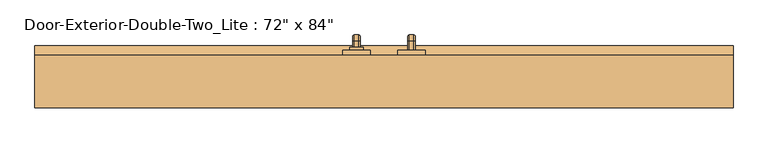
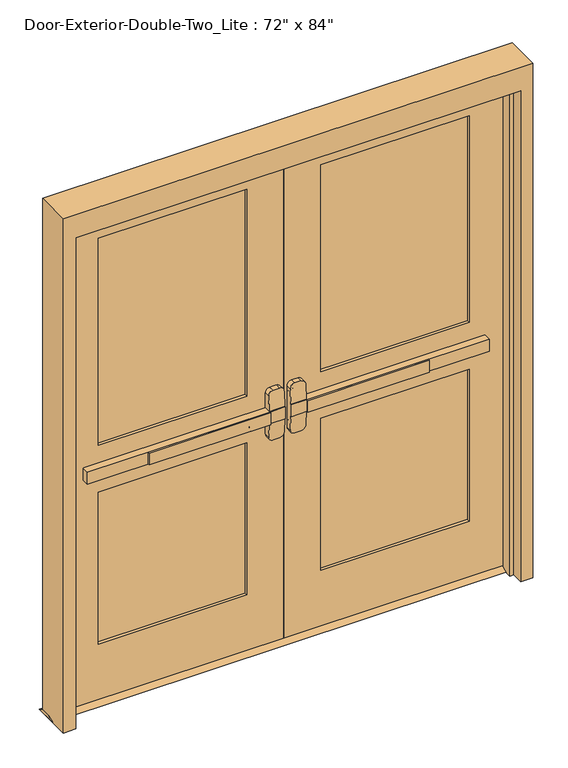
"""IFC4 building model written with IfcOpenShell, lengths in millimetres: door geometry."""

from ifc_helpers import new_model, si_unit, point, frame, frame_2d, origin, place, context, project, spatial, polyline, circle_curve, ellipse_curve, trimmed, segment, composite_curve, outline, extrude, faceted_brep, source, transform, mapped, element, save
from ifc_brep_helpers import plane_surface, cylinder_surface, revolved_surface, advanced_brep


def door_6260e01d(model_context):
    return source(origin(), model_context, "Body", "SolidModel", [
        extrude(outline(polyline([(-575.7333333, 0.0), (-575.7333333, 6.35), (-76.2, 6.35), (-76.2, 0.0), (-575.7333333, 0.0)])), frame((0.0, 0.0, 990.6), z_axis=(0.0, 0.0, 1.0), x_axis=(1.0, 0.0, 0.0)), (0.0, 0.0, 1.0), 50.8),
        advanced_brep(
        [(-12.7, 6.35, 1041.4), (-76.2, 6.35, 1041.4), (-825.5, 6.35, 1041.4), (-825.5, 6.35, 990.6), (-76.2, 6.35, 990.6), (-12.7, 6.35, 990.6), (-825.5, 38.1, 1041.4), (-76.2, 38.1, 1041.4), (-76.2, 38.1, 1104.9), (-57.15, 38.1, 1123.95), (-31.75, 38.1, 1123.95), (-12.7, 38.1, 1104.9), (-12.7, 38.1, 927.1), (-31.75, 38.1, 908.05), (-57.15, 38.1, 908.05), (-76.2, 38.1, 927.1), (-76.2, 38.1, 990.6), (-825.5, 38.1, 990.6), (-12.7, 9.5252467, 1041.4), (-76.2, 9.5252467, 1041.4), (-12.7, 9.5252467, 990.6), (-12.7, 14.5354269, 927.1), (-12.7, 14.5354269, 1104.9), (-76.2, 9.5252467, 990.6), (-76.2, 14.5354269, 1104.9), (-76.2, 14.5354269, 927.1), (-57.15, 16.038481, 1123.95), (-31.75, 16.038481, 1123.95), (-31.75, 16.038481, 908.05), (-57.15, 16.038481, 908.05)],
        [
            (0, 1),
            (1, 2),
            (2, 3),
            (3, 4),
            (4, 5),
            (5, 0),
            (6, 7),
            (7, 8),
            (8, 9, circle_curve(frame((-57.15, 38.1, 1104.9), z_axis=(0.0, 1.0, 0.0), x_axis=(-1.0, 0.0, 0.0)), 19.05)),
            (9, 10),
            (10, 11, circle_curve(frame((-31.75, 38.1, 1104.9), z_axis=(0.0, 1.0, 0.0), x_axis=(-1.0, 0.0, 0.0)), 19.05)),
            (11, 12),
            (12, 13, circle_curve(frame((-31.75, 38.1, 927.1), z_axis=(0.0, 1.0, 0.0), x_axis=(-1.0, 0.0, 0.0)), 19.05)),
            (13, 14),
            (14, 15, circle_curve(frame((-57.15, 38.1, 927.1), z_axis=(0.0, 1.0, 0.0), x_axis=(-1.0, 0.0, 0.0)), 19.05)),
            (15, 16),
            (16, 17),
            (17, 6),
            (0, 18),
            (18, 19),
            (19, 7),
            (6, 2),
            (5, 20),
            (20, 21),
            (21, 12),
            (11, 22),
            (22, 18),
            (16, 23),
            (23, 20),
            (3, 17),
            (19, 24),
            (24, 8),
            (15, 25),
            (25, 23),
            (9, 26),
            (26, 27),
            (27, 10),
            (13, 28),
            (28, 29),
            (29, 14),
            (29, 25, ellipse_curve(frame((-57.15, 14.5354269, 927.1), z_axis=(0.0, 0.9969018152893365, 0.07865602756830282), x_axis=(0.0, -0.07865602756830208, 0.9969018152893365)), 19.1092038, 19.05)),
            (24, 26, ellipse_curve(frame((-57.15, 14.5354269, 1104.9), z_axis=(0.0, 0.9969018152893376, -0.07865602756828934), x_axis=(0.0, -0.078656027568288, -0.9969018152893377)), 19.1092038, 19.05)),
            (27, 22, ellipse_curve(frame((-31.75, 14.5354269, 1104.9), z_axis=(0.0, 0.9969018152893376, -0.07865602756828934), x_axis=(0.0, -0.078656027568288, -0.9969018152893377)), 19.1092038, 19.05)),
            (21, 28, ellipse_curve(frame((-31.75, 14.5354269, 927.1), z_axis=(0.0, 0.9969018152893365, 0.07865602756830282), x_axis=(0.0, -0.07865602756830208, 0.9969018152893365)), 19.1092038, 19.05)),
        ],
        [
            plane_surface(frame((-12.7, 6.35, 1041.4), z_axis=(0.0, -1.0, 0.0), x_axis=(1.0, 0.0, 0.0))),
            plane_surface(frame((-12.7, 38.1, 1041.4), z_axis=(0.0, 1.0, 0.0), x_axis=(-1.0, 0.0, 0.0))),
            plane_surface(frame((-825.5, 6.35, 1041.4), z_axis=(0.0, 0.0, 1.0), x_axis=(0.0, 1.0, 0.0))),
            plane_surface(frame((-12.7, 6.35, 1041.4), z_axis=(1.0, 0.0, 0.0), x_axis=(0.0, 1.0, 0.0))),
            plane_surface(frame((-12.7, 6.35, 990.6), z_axis=(0.0, 0.0, -1.0), x_axis=(0.0, 1.0, 0.0))),
            plane_surface(frame((-825.5, 6.35, 990.6), z_axis=(-1.0, 0.0, 0.0), x_axis=(0.0, 1.0, 0.0))),
            plane_surface(frame((-76.2, 9.5252467, 927.1), z_axis=(-1.0, 0.0, 0.0), x_axis=(0.0, 1.0, 0.0))),
            plane_surface(frame((-57.15, 9.5252467, 1123.95), z_axis=(0.0, 0.0, 1.0), x_axis=(0.0, 1.0, 0.0))),
            plane_surface(frame((-31.75, 9.5252467, 908.05), z_axis=(0.0, 0.0, -1.0), x_axis=(0.0, 1.0, 0.0))),
            cylinder_surface(frame((-57.15, 38.1, 927.1), z_axis=(0.0, -1.0, 0.0), x_axis=(-1.0, 0.0, 0.0)), 19.05),
            cylinder_surface(frame((-57.15, 38.1, 1104.9), z_axis=(0.0, -1.0, 0.0), x_axis=(-1.0, 0.0, 0.0)), 19.05),
            cylinder_surface(frame((-31.75, 38.1, 1104.9), z_axis=(0.0, -1.0, 0.0), x_axis=(-1.0, 0.0, 0.0)), 19.05),
            cylinder_surface(frame((-31.75, 38.1, 927.1), z_axis=(0.0, -1.0, 0.0), x_axis=(-1.0, 0.0, 0.0)), 19.05),
            plane_surface(frame((-76.2, 9.5252467, 1041.4), z_axis=(0.0, -0.9969018152893376, 0.07865602756828934), x_axis=(1.0, 0.0, 0.0))),
            plane_surface(frame((-76.2, 16.038481, 908.05), z_axis=(0.0, -0.9969018152893365, -0.07865602756830282), x_axis=(1.0, 0.0, 0.0))),
        ],
        [
            (0, [[1, 2, 3, 4, 5, 6]]),
            (1, [[7, 8, 9, 10, 11, 12, 13, 14, 15, 16, 17, 18]]),
            (2, [[-2, -1, 19, 20, 21, -7, 22]]),
            (3, [[23, 24, 25, -12, 26, 27, -19, -6]]),
            (4, [[-17, 28, 29, -23, -5, -4, 30]]),
            (5, [[-22, -18, -30, -3]]),
            (6, [[-21, 31, 32, -8]]),
            (6, [[33, 34, -28, -16]]),
            (7, [[35, 36, 37, -10]]),
            (8, [[38, 39, 40, -14]]),
            (9, [[-40, 41, -33, -15]]),
            (10, [[-32, 42, -35, -9]]),
            (11, [[-37, 43, -26, -11]]),
            (12, [[-25, 44, -38, -13]]),
            (13, [[-27, -43, -36, -42, -31, -20]]),
            (14, [[-29, -34, -41, -39, -44, -24]]),
        ],
    ),
        extrude(outline(polyline([(82.55, 12.7), (107.95, 0.0), (12.7, 0.0), (38.1, 12.7), (82.55, 12.7)])), frame((-965.2, 0.0, 0.0), z_axis=(1.0, 0.0, 0.0), x_axis=(0.0, 1.0, 0.0)), (0.0, 0.0, 1.0), 1930.4),
        extrude(outline(polyline([(575.7333333, 0.0), (76.2, 0.0), (76.2, 6.35), (575.7333333, 6.35), (575.7333333, 0.0)])), frame((0.0, 0.0, 990.6), z_axis=(0.0, 0.0, 1.0), x_axis=(1.0, 0.0, 0.0)), (0.0, 0.0, 1.0), 50.8),
        advanced_brep(
        [(12.7, 6.35, 1041.4), (12.7, 6.35, 990.6), (76.2, 6.35, 990.6), (825.5, 6.35, 990.6), (825.5, 6.35, 1041.4), (76.2, 6.35, 1041.4), (825.5, 38.1, 1041.4), (825.5, 38.1, 990.6), (76.2, 38.1, 990.6), (76.2, 38.1, 927.1), (57.15, 38.1, 908.05), (31.75, 38.1, 908.05), (12.7, 38.1, 927.1), (12.7, 38.1, 1104.9), (31.75, 38.1, 1123.95), (57.15, 38.1, 1123.95), (76.2, 38.1, 1104.9), (76.2, 38.1, 1041.4), (76.2, 9.5252467, 1041.4), (12.7, 9.5252467, 1041.4), (12.7, 14.5354269, 1104.9), (12.7, 14.5354269, 927.1), (12.7, 9.5252467, 990.6), (76.2, 9.5252467, 990.6), (76.2, 14.5354269, 927.1), (76.2, 14.5354269, 1104.9), (31.75, 16.038481, 1123.95), (57.15, 16.038481, 1123.95), (57.15, 16.038481, 908.05), (31.75, 16.038481, 908.05)],
        [
            (0, 1),
            (1, 2),
            (2, 3),
            (3, 4),
            (4, 5),
            (5, 0),
            (6, 7),
            (7, 8),
            (8, 9),
            (9, 10, circle_curve(frame((57.15, 38.1, 927.1), z_axis=(0.0, 1.0, 0.0), x_axis=(1.0, 0.0, 0.0)), 19.05)),
            (10, 11),
            (11, 12, circle_curve(frame((31.75, 38.1, 927.1), z_axis=(0.0, 1.0, 0.0), x_axis=(1.0, 0.0, 0.0)), 19.05)),
            (12, 13),
            (13, 14, circle_curve(frame((31.75, 38.1, 1104.9), z_axis=(0.0, 1.0, 0.0), x_axis=(1.0, 0.0, 0.0)), 19.05)),
            (14, 15),
            (15, 16, circle_curve(frame((57.15, 38.1, 1104.9), z_axis=(0.0, 1.0, 0.0), x_axis=(1.0, 0.0, 0.0)), 19.05)),
            (16, 17),
            (17, 6),
            (4, 6),
            (17, 18),
            (18, 19),
            (19, 0),
            (19, 20),
            (20, 13),
            (12, 21),
            (21, 22),
            (22, 1),
            (7, 3),
            (22, 23),
            (23, 8),
            (23, 24),
            (24, 9),
            (16, 25),
            (25, 18),
            (14, 26),
            (26, 27),
            (27, 15),
            (10, 28),
            (28, 29),
            (29, 11),
            (24, 28, ellipse_curve(frame((57.15, 14.5354269, 927.1), z_axis=(0.0, 0.9969018152893365, 0.07865602756830282), x_axis=(0.0, -0.07865602756830208, 0.9969018152893365)), 19.1092038, 19.05)),
            (27, 25, ellipse_curve(frame((57.15, 14.5354269, 1104.9), z_axis=(0.0, 0.9969018152893376, -0.07865602756828934), x_axis=(0.0, -0.078656027568288, -0.9969018152893377)), 19.1092038, 19.05)),
            (20, 26, ellipse_curve(frame((31.75, 14.5354269, 1104.9), z_axis=(0.0, 0.9969018152893376, -0.07865602756828934), x_axis=(0.0, -0.078656027568288, -0.9969018152893377)), 19.1092038, 19.05)),
            (29, 21, ellipse_curve(frame((31.75, 14.5354269, 927.1), z_axis=(0.0, 0.9969018152893365, 0.07865602756830282), x_axis=(0.0, -0.07865602756830208, 0.9969018152893365)), 19.1092038, 19.05)),
        ],
        [
            plane_surface(frame((12.7, 6.35, 1041.4), z_axis=(0.0, -1.0, 0.0), x_axis=(-1.0, 0.0, 0.0))),
            plane_surface(frame((12.7, 38.1, 1041.4), z_axis=(0.0, 1.0, 0.0), x_axis=(1.0, 0.0, 0.0))),
            plane_surface(frame((825.5, 6.35, 1041.4), z_axis=(0.0, 0.0, 1.0), x_axis=(0.0, 1.0, 0.0))),
            plane_surface(frame((12.7, 6.35, 1041.4), z_axis=(-1.0, 0.0, 0.0), x_axis=(0.0, 1.0, 0.0))),
            plane_surface(frame((12.7, 6.35, 990.6), z_axis=(0.0, 0.0, -1.0), x_axis=(0.0, 1.0, 0.0))),
            plane_surface(frame((825.5, 6.35, 990.6), z_axis=(1.0, 0.0, 0.0), x_axis=(0.0, 1.0, 0.0))),
            plane_surface(frame((76.2, 9.5252467, 927.1), z_axis=(1.0, 0.0, 0.0), x_axis=(0.0, 1.0, 0.0))),
            plane_surface(frame((57.15, 9.5252467, 1123.95), z_axis=(0.0, 0.0, 1.0), x_axis=(0.0, 1.0, 0.0))),
            plane_surface(frame((31.75, 9.5252467, 908.05), z_axis=(0.0, 0.0, -1.0), x_axis=(0.0, 1.0, 0.0))),
            cylinder_surface(frame((57.15, 38.1, 927.1), z_axis=(0.0, -1.0, 0.0), x_axis=(1.0, 0.0, 0.0)), 19.05),
            cylinder_surface(frame((57.15, 38.1, 1104.9), z_axis=(0.0, -1.0, 0.0), x_axis=(1.0, 0.0, 0.0)), 19.05),
            cylinder_surface(frame((31.75, 38.1, 1104.9), z_axis=(0.0, -1.0, 0.0), x_axis=(1.0, 0.0, 0.0)), 19.05),
            cylinder_surface(frame((31.75, 38.1, 927.1), z_axis=(0.0, -1.0, 0.0), x_axis=(1.0, 0.0, 0.0)), 19.05),
            plane_surface(frame((76.2, 9.5252467, 1041.4), z_axis=(0.0, -0.9969018152893376, 0.07865602756828934), x_axis=(-1.0, 0.0, 0.0))),
            plane_surface(frame((76.2, 16.038481, 908.05), z_axis=(0.0, -0.9969018152893365, -0.07865602756830282), x_axis=(-1.0, 0.0, 0.0))),
        ],
        [
            (0, [[1, 2, 3, 4, 5, 6]]),
            (1, [[7, 8, 9, 10, 11, 12, 13, 14, 15, 16, 17, 18]]),
            (2, [[19, -18, 20, 21, 22, -6, -5]]),
            (3, [[-1, -22, 23, 24, -13, 25, 26, 27]]),
            (4, [[28, -3, -2, -27, 29, 30, -8]]),
            (5, [[-4, -28, -7, -19]]),
            (6, [[-9, -30, 31, 32]]),
            (6, [[-17, 33, 34, -20]]),
            (7, [[-15, 35, 36, 37]]),
            (8, [[-11, 38, 39, 40]]),
            (9, [[-10, -32, 41, -38]]),
            (10, [[-16, -37, 42, -33]]),
            (11, [[-14, -24, 43, -35]]),
            (12, [[-12, -40, 44, -25]]),
            (13, [[-21, -34, -42, -36, -43, -23]]),
            (14, [[-26, -44, -39, -41, -31, -29]]),
        ],
    ),
        advanced_brep(
        [(66.2, 95.25, 1017.190625), (66.2, 95.25, 1014.809375), (69.771875, 95.25, 1011.2375), (82.6284594, 95.25, 1011.2375), (86.2, 95.25, 1014.8090406), (86.2, 95.25, 1017.190625), (82.628125, 95.25, 1020.7625), (69.771875, 95.25, 1020.7625), (66.2, 95.25, 887.809375), (69.771875, 95.25, 884.2375), (82.628125, 95.25, 884.2375), (86.2, 95.25, 887.809375), (86.2, 95.25, 890.1909594), (82.6284594, 95.25, 893.7625), (69.771875, 95.25, 893.7625), (66.2, 95.25, 890.190625), (66.2, 120.65, 1017.190625), (66.2, 134.540625, 1003.3), (66.2, 134.540625, 901.7), (66.2, 120.65, 887.809375), (66.2, 120.65, 890.190625), (66.2, 132.159375, 901.7), (66.2, 132.159375, 1003.3), (66.2, 120.65, 1014.809375), (69.771875, 120.65, 1011.2375), (82.6284594, 120.65, 1011.2375), (86.2, 120.65, 1014.8090406), (86.2, 132.1590406, 1003.3), (86.2, 132.1590406, 901.7), (86.2, 120.65, 890.1909594), (86.2, 120.65, 887.809375), (86.2, 134.540625, 901.7), (86.2, 134.540625, 1003.3), (86.2, 120.65, 1017.190625), (82.628125, 120.65, 1020.7625), (69.771875, 120.65, 1020.7625), (69.771875, 128.5875, 1003.3), (82.6284594, 128.5875, 1003.3), (82.628125, 138.1125, 1003.3), (69.771875, 138.1125, 1003.3), (69.771875, 128.5875, 901.7), (82.6284594, 128.5875, 901.7), (82.628125, 138.1125, 901.7), (69.771875, 138.1125, 901.7), (69.771875, 120.65, 893.7625), (82.6284594, 120.65, 893.7625), (82.628125, 120.65, 884.2375), (69.771875, 120.65, 884.2375)],
        [
            (0, 1),
            (1, 2, circle_curve(frame((69.771875, 95.25, 1014.809375), z_axis=(0.0, -1.0, 0.0), x_axis=(0.0, 0.0, 1.0)), 3.571875)),
            (2, 3),
            (3, 4, circle_curve(frame((82.6284594, 95.25, 1014.8090406), z_axis=(0.0, -1.0, 0.0), x_axis=(0.0, 0.0, 1.0)), 3.5715406)),
            (4, 5),
            (5, 6, circle_curve(frame((82.628125, 95.25, 1017.190625), z_axis=(0.0, -1.0, 0.0), x_axis=(0.0, 0.0, 1.0)), 3.571875)),
            (6, 7),
            (7, 0, circle_curve(frame((69.771875, 95.25, 1017.190625), z_axis=(0.0, -1.0, 0.0), x_axis=(0.0, 0.0, 1.0)), 3.571875)),
            (8, 9, circle_curve(frame((69.771875, 95.25, 887.809375), z_axis=(0.0, -1.0, 0.0), x_axis=(0.0, 0.0, -1.0)), 3.571875)),
            (9, 10),
            (10, 11, circle_curve(frame((82.628125, 95.25, 887.809375), z_axis=(0.0, -1.0, 0.0), x_axis=(0.0, 0.0, -1.0)), 3.571875)),
            (11, 12),
            (12, 13, circle_curve(frame((82.6284594, 95.25, 890.1909594), z_axis=(0.0, -1.0, 0.0), x_axis=(0.0, 0.0, -1.0)), 3.5715406)),
            (13, 14),
            (14, 15, circle_curve(frame((69.771875, 95.25, 890.190625), z_axis=(0.0, -1.0, 0.0), x_axis=(0.0, 0.0, -1.0)), 3.571875)),
            (15, 8),
            (0, 16),
            (16, 17, circle_curve(frame((66.2, 120.65, 1003.3), z_axis=(-1.0, 0.0, 0.0), x_axis=(0.0, 0.0, 1.0)), 13.890625)),
            (17, 18),
            (18, 19, circle_curve(frame((66.2, 120.65, 901.7), z_axis=(-1.0, 0.0, 0.0), x_axis=(0.0, 1.0, 0.0)), 13.890625)),
            (19, 8),
            (15, 20),
            (20, 21, circle_curve(frame((66.2, 120.65, 901.7), z_axis=(1.0, 0.0, 0.0), x_axis=(0.0, 1.0, 0.0)), 11.509375)),
            (21, 22),
            (22, 23, circle_curve(frame((66.2, 120.65, 1003.3), z_axis=(1.0, 0.0, 0.0), x_axis=(0.0, 0.0, 1.0)), 11.509375)),
            (23, 1),
            (23, 24, circle_curve(frame((69.771875, 120.65, 1014.809375), z_axis=(0.0, -1.0, 0.0), x_axis=(0.0, 0.0, 1.0)), 3.571875)),
            (24, 2),
            (24, 25),
            (25, 3),
            (25, 26, circle_curve(frame((82.6284594, 120.65, 1014.8090406), z_axis=(0.0, -1.0, 0.0), x_axis=(0.0, 0.0, 1.0)), 3.5715406)),
            (26, 4),
            (26, 27, circle_curve(frame((86.2, 120.65, 1003.3), z_axis=(-1.0, 0.0, 0.0), x_axis=(0.0, 0.0, 1.0)), 11.5090406)),
            (27, 28),
            (28, 29, circle_curve(frame((86.2, 120.65, 901.7), z_axis=(-1.0, 0.0, 0.0), x_axis=(0.0, 1.0, 0.0)), 11.5090406)),
            (29, 12),
            (11, 30),
            (30, 31, circle_curve(frame((86.2, 120.65, 901.7), z_axis=(1.0, 0.0, 0.0), x_axis=(0.0, 1.0, 0.0)), 13.890625)),
            (31, 32),
            (32, 33, circle_curve(frame((86.2, 120.65, 1003.3), z_axis=(1.0, 0.0, 0.0), x_axis=(0.0, 0.0, 1.0)), 13.890625)),
            (33, 5),
            (33, 34, circle_curve(frame((82.628125, 120.65, 1017.190625), z_axis=(0.0, -1.0, 0.0), x_axis=(0.0, 0.0, 1.0)), 3.571875)),
            (34, 6),
            (34, 35),
            (35, 7),
            (35, 16, circle_curve(frame((69.771875, 120.65, 1017.190625), z_axis=(0.0, -1.0, 0.0), x_axis=(0.0, 0.0, 1.0)), 3.571875)),
            (36, 24, circle_curve(frame((69.771875, 120.65, 1003.3), z_axis=(1.0, 0.0, 0.0), x_axis=(0.0, 0.0, 1.0)), 7.9375)),
            (22, 36, circle_curve(frame((69.771875, 132.159375, 1003.3), z_axis=(0.0, 0.0, 1.0), x_axis=(0.0, 1.0, 0.0)), 3.571875)),
            (37, 25, circle_curve(frame((82.6284594, 120.65, 1003.3), z_axis=(1.0, 0.0, 0.0), x_axis=(0.0, 0.0, 1.0)), 7.9375)),
            (36, 37),
            (37, 27, circle_curve(frame((82.6284594, 132.1590406, 1003.3), z_axis=(0.0, 0.0, 1.0), x_axis=(0.0, 1.0, 0.0)), 3.5715406)),
            (38, 34, circle_curve(frame((82.628125, 120.65, 1003.3), z_axis=(1.0, 0.0, 0.0), x_axis=(0.0, 0.0, 1.0)), 17.4625)),
            (32, 38, circle_curve(frame((82.628125, 134.540625, 1003.3), z_axis=(0.0, 0.0, 1.0), x_axis=(0.0, 1.0, 0.0)), 3.571875)),
            (39, 35, circle_curve(frame((69.771875, 120.65, 1003.3), z_axis=(1.0, 0.0, 0.0), x_axis=(0.0, 0.0, 1.0)), 17.4625)),
            (38, 39),
            (39, 17, circle_curve(frame((69.771875, 134.540625, 1003.3), z_axis=(0.0, 0.0, 1.0), x_axis=(0.0, 1.0, 0.0)), 3.571875)),
            (21, 40, circle_curve(frame((69.771875, 132.159375, 901.7), z_axis=(0.0, 0.0, 1.0), x_axis=(0.0, 1.0, 0.0)), 3.571875)),
            (40, 36),
            (40, 41),
            (41, 37),
            (41, 28, circle_curve(frame((82.6284594, 132.1590406, 901.7), z_axis=(0.0, 0.0, 1.0), x_axis=(0.0, 1.0, 0.0)), 3.5715406)),
            (31, 42, circle_curve(frame((82.628125, 134.540625, 901.7), z_axis=(0.0, 0.0, 1.0), x_axis=(0.0, 1.0, 0.0)), 3.571875)),
            (42, 38),
            (42, 43),
            (43, 39),
            (43, 18, circle_curve(frame((69.771875, 134.540625, 901.7), z_axis=(0.0, 0.0, 1.0), x_axis=(0.0, 1.0, 0.0)), 3.571875)),
            (44, 40, circle_curve(frame((69.771875, 120.65, 901.7), z_axis=(1.0, 0.0, 0.0), x_axis=(0.0, 1.0, 0.0)), 7.9375)),
            (20, 44, circle_curve(frame((69.771875, 120.65, 890.190625), z_axis=(0.0, 1.0, 0.0), x_axis=(0.0, 0.0, -1.0)), 3.571875)),
            (45, 41, circle_curve(frame((82.6284594, 120.65, 901.7), z_axis=(1.0, 0.0, 0.0), x_axis=(0.0, 1.0, 0.0)), 7.9375)),
            (44, 45),
            (45, 29, circle_curve(frame((82.6284594, 120.65, 890.1909594), z_axis=(0.0, 1.0, 0.0), x_axis=(0.0, 0.0, -1.0)), 3.5715406)),
            (46, 42, circle_curve(frame((82.628125, 120.65, 901.7), z_axis=(1.0, 0.0, 0.0), x_axis=(0.0, 1.0, 0.0)), 17.4625)),
            (30, 46, circle_curve(frame((82.628125, 120.65, 887.809375), z_axis=(0.0, 1.0, 0.0), x_axis=(0.0, 0.0, -1.0)), 3.571875)),
            (47, 43, circle_curve(frame((69.771875, 120.65, 901.7), z_axis=(1.0, 0.0, 0.0), x_axis=(0.0, 1.0, 0.0)), 17.4625)),
            (46, 47),
            (47, 19, circle_curve(frame((69.771875, 120.65, 887.809375), z_axis=(0.0, 1.0, 0.0), x_axis=(0.0, 0.0, -1.0)), 3.571875)),
            (14, 44),
            (13, 45),
            (10, 46),
            (9, 47),
        ],
        [
            plane_surface(frame((76.2, 95.25, 1016.0), z_axis=(0.0, -1.0, 0.0), x_axis=(1.0, 0.0, 0.0))),
            plane_surface(frame((76.2, 95.25, 889.0), z_axis=(0.0, -1.0, 0.0), x_axis=(1.0, 0.0, 0.0))),
            plane_surface(frame((66.2, 95.25, 1017.190625), z_axis=(-1.0, 0.0, 0.0), x_axis=(0.0, 1.0, 0.0))),
            cylinder_surface(frame((69.771875, 95.25, 1014.809375), z_axis=(0.0, -1.0, 0.0), x_axis=(0.0, 0.0, 1.0)), 3.571875),
            plane_surface(frame((69.771875, 95.25, 1011.2375), z_axis=(0.0, 0.0, -1.0), x_axis=(0.0, 1.0, 0.0))),
            cylinder_surface(frame((82.6284594, 95.25, 1014.8090406), z_axis=(0.0, -1.0, 0.0), x_axis=(0.0, 0.0, 1.0)), 3.5715406),
            plane_surface(frame((86.2, 95.25, 1014.8090406), z_axis=(1.0, 0.0, 0.0), x_axis=(0.0, 1.0, 0.0))),
            cylinder_surface(frame((82.628125, 95.25, 1017.190625), z_axis=(0.0, -1.0, 0.0), x_axis=(0.0, 0.0, 1.0)), 3.571875),
            plane_surface(frame((82.628125, 95.25, 1020.7625), z_axis=(0.0, 0.0, 1.0), x_axis=(0.0, 1.0, 0.0))),
            cylinder_surface(frame((69.771875, 95.25, 1017.190625), z_axis=(0.0, -1.0, 0.0), x_axis=(0.0, 0.0, 1.0)), 3.571875),
            revolved_surface(trimmed(ellipse_curve(frame((69.771875, 120.65, 1014.809375), z_axis=(0.0, -1.0, 0.0), x_axis=(0.0, 0.0, 1.0)), 3.571875, 3.571875), [point((66.2, 120.65, 1014.809375))], [point((69.771875, 120.65, 1011.2375))], True, "CARTESIAN"), (76.2, 120.65, 1003.3), (-1.0, 0.0, 0.0)),
            revolved_surface(polyline([(69.771875, 120.65, 1011.2375), (82.6284594, 120.65, 1011.2375)]), (76.2, 120.65, 1003.3), (-1.0, 0.0, 0.0)),
            revolved_surface(trimmed(ellipse_curve(frame((82.6284594, 120.65, 1014.8090406), z_axis=(0.0, -1.0, 0.0), x_axis=(0.0, 0.0, 1.0)), 3.5715406, 3.5715406), [point((82.6284594, 120.65, 1011.2375))], [point((86.2, 120.65, 1014.8090406))], True, "CARTESIAN"), (76.2, 120.65, 1003.3), (-1.0, 0.0, 0.0)),
            revolved_surface(trimmed(ellipse_curve(frame((82.628125, 120.65, 1017.190625), z_axis=(0.0, -1.0, 0.0), x_axis=(0.0, 0.0, 1.0)), 3.571875, 3.571875), [point((86.2, 120.65, 1017.190625))], [point((82.628125, 120.65, 1020.7625))], True, "CARTESIAN"), (76.2, 120.65, 1003.3), (-1.0, 0.0, 0.0)),
            cylinder_surface(frame((76.2, 120.65, 1003.3), z_axis=(-1.0, 0.0, 0.0), x_axis=(0.0, 0.0, 1.0)), 17.4625),
            revolved_surface(trimmed(ellipse_curve(frame((69.771875, 120.65, 1017.190625), z_axis=(0.0, -1.0, 0.0), x_axis=(0.0, 0.0, 1.0)), 3.571875, 3.571875), [point((69.771875, 120.65, 1020.7625))], [point((66.2, 120.65, 1017.190625))], True, "CARTESIAN"), (76.2, 120.65, 1003.3), (-1.0, 0.0, 0.0)),
            cylinder_surface(frame((69.771875, 132.159375, 1003.3), z_axis=(0.0, 0.0, 1.0), x_axis=(0.0, 1.0, 0.0)), 3.571875),
            plane_surface(frame((69.771875, 128.5875, 1003.3), z_axis=(0.0, -1.0, 0.0), x_axis=(0.0, 0.0, -1.0))),
            cylinder_surface(frame((82.6284594, 132.1590406, 1003.3), z_axis=(0.0, 0.0, 1.0), x_axis=(0.0, 1.0, 0.0)), 3.5715406),
            cylinder_surface(frame((82.628125, 134.540625, 1003.3), z_axis=(0.0, 0.0, 1.0), x_axis=(0.0, 1.0, 0.0)), 3.571875),
            plane_surface(frame((82.628125, 138.1125, 1003.3), z_axis=(0.0, 1.0, 0.0), x_axis=(0.0, 0.0, -1.0))),
            cylinder_surface(frame((69.771875, 134.540625, 1003.3), z_axis=(0.0, 0.0, 1.0), x_axis=(0.0, 1.0, 0.0)), 3.571875),
            revolved_surface(trimmed(ellipse_curve(frame((69.771875, 132.159375, 901.7), z_axis=(0.0, 0.0, 1.0), x_axis=(0.0, 1.0, 0.0)), 3.571875, 3.571875), [point((66.2, 132.159375, 901.7))], [point((69.771875, 128.5875, 901.7))], True, "CARTESIAN"), (76.2, 120.65, 901.7), (-1.0, 0.0, 0.0)),
            revolved_surface(polyline([(69.771875, 128.5875, 901.7), (82.6284594, 128.5875, 901.7)]), (76.2, 120.65, 901.7), (-1.0, 0.0, 0.0)),
            revolved_surface(trimmed(ellipse_curve(frame((82.6284594, 132.1590406, 901.7), z_axis=(0.0, 0.0, 1.0), x_axis=(0.0, 1.0, 0.0)), 3.5715406, 3.5715406), [point((82.6284594, 128.5875, 901.7))], [point((86.2, 132.1590406, 901.7))], True, "CARTESIAN"), (76.2, 120.65, 901.7), (-1.0, 0.0, 0.0)),
            revolved_surface(trimmed(ellipse_curve(frame((82.628125, 134.540625, 901.7), z_axis=(0.0, 0.0, 1.0), x_axis=(0.0, 1.0, 0.0)), 3.571875, 3.571875), [point((86.2, 134.540625, 901.7))], [point((82.628125, 138.1125, 901.7))], True, "CARTESIAN"), (76.2, 120.65, 901.7), (-1.0, 0.0, 0.0)),
            cylinder_surface(frame((76.2, 120.65, 901.7), z_axis=(-1.0, 0.0, 0.0), x_axis=(0.0, 1.0, 0.0)), 17.4625),
            revolved_surface(trimmed(ellipse_curve(frame((69.771875, 134.540625, 901.7), z_axis=(0.0, 0.0, 1.0), x_axis=(0.0, 1.0, 0.0)), 3.571875, 3.571875), [point((69.771875, 138.1125, 901.7))], [point((66.2, 134.540625, 901.7))], True, "CARTESIAN"), (76.2, 120.65, 901.7), (-1.0, 0.0, 0.0)),
            cylinder_surface(frame((69.771875, 120.65, 890.190625), z_axis=(0.0, 1.0, 0.0), x_axis=(0.0, 0.0, -1.0)), 3.571875),
            plane_surface(frame((69.771875, 120.65, 893.7625), z_axis=(0.0, 0.0, 1.0), x_axis=(0.0, -1.0, 0.0))),
            cylinder_surface(frame((82.6284594, 120.65, 890.1909594), z_axis=(0.0, 1.0, 0.0), x_axis=(0.0, 0.0, -1.0)), 3.5715406),
            cylinder_surface(frame((82.628125, 120.65, 887.809375), z_axis=(0.0, 1.0, 0.0), x_axis=(0.0, 0.0, -1.0)), 3.571875),
            plane_surface(frame((82.628125, 120.65, 884.2375), z_axis=(0.0, 0.0, -1.0), x_axis=(0.0, -1.0, 0.0))),
            cylinder_surface(frame((69.771875, 120.65, 887.809375), z_axis=(0.0, 1.0, 0.0), x_axis=(0.0, 0.0, -1.0)), 3.571875),
        ],
        [
            (0, [[1, 2, 3, 4, 5, 6, 7, 8]]),
            (1, [[9, 10, 11, 12, 13, 14, 15, 16]]),
            (2, [[-1, 17, 18, 19, 20, 21, -16, 22, 23, 24, 25, 26]]),
            (3, [[-2, -26, 27, 28]]),
            (4, [[-3, -28, 29, 30]]),
            (5, [[-4, -30, 31, 32]]),
            (6, [[-5, -32, 33, 34, 35, 36, -12, 37, 38, 39, 40, 41]]),
            (7, [[-6, -41, 42, 43]]),
            (8, [[-7, -43, 44, 45]]),
            (9, [[-8, -45, 46, -17]]),
            (10, [[47, -27, -25, 48]]),
            (11, [[49, -29, -47, 50]]),
            (12, [[-33, -31, -49, 51]]),
            (13, [[52, -42, -40, 53]]),
            (14, [[54, -44, -52, 55]]),
            (15, [[-18, -46, -54, 56]]),
            (16, [[-48, -24, 57, 58]]),
            (17, [[-50, -58, 59, 60]]),
            (18, [[-51, -60, 61, -34]]),
            (19, [[-53, -39, 62, 63]]),
            (20, [[-55, -63, 64, 65]]),
            (21, [[-56, -65, 66, -19]]),
            (22, [[67, -57, -23, 68]]),
            (23, [[69, -59, -67, 70]]),
            (24, [[-35, -61, -69, 71]]),
            (25, [[72, -62, -38, 73]]),
            (26, [[74, -64, -72, 75]]),
            (27, [[-20, -66, -74, 76]]),
            (28, [[-68, -22, -15, 77]]),
            (29, [[-70, -77, -14, 78]]),
            (30, [[-71, -78, -13, -36]]),
            (31, [[-73, -37, -11, 79]]),
            (32, [[-75, -79, -10, 80]]),
            (33, [[-76, -80, -9, -21]]),
        ],
    ),
        extrude(outline(composite_curve([segment(trimmed(circle_curve(frame_2d((1113.0338574, 76.2)), 89.3016225), [point((1193.8, 114.3))], [point((1193.8, 38.1))], False, "CARTESIAN"), True, "CONTINUOUS"), segment(polyline([(1193.8, 38.1), (838.2, 38.1)]), True, "CONTINUOUS"), segment(trimmed(circle_curve(frame_2d((918.9661426, 76.2)), 89.3016225), [point((838.2, 38.1))], [point((838.2, 114.3))], False, "CARTESIAN"), True, "CONTINUOUS"), segment(polyline([(838.2, 114.3), (1193.8, 114.3)]), True, "CONTINUOUS")], self_intersect=False)), frame((0.0, 82.55, 0.0), z_axis=(0.0, 1.0, 0.0), x_axis=(0.0, 0.0, 1.0)), (0.0, 0.0, 1.0), 12.7),
        advanced_brep(
        [(-86.2, 95.25, 1017.190625), (-86.2, 95.25, 1014.809375), (-82.628125, 95.25, 1011.2375), (-69.7715406, 95.25, 1011.2375), (-66.2, 95.25, 1014.8090406), (-66.2, 95.25, 1017.190625), (-69.771875, 95.25, 1020.7625), (-82.628125, 95.25, 1020.7625), (-86.2, 95.25, 887.809375), (-82.628125, 95.25, 884.2375), (-69.771875, 95.25, 884.2375), (-66.2, 95.25, 887.809375), (-66.2, 95.25, 890.1909594), (-69.7715406, 95.25, 893.7625), (-82.628125, 95.25, 893.7625), (-86.2, 95.25, 890.190625), (-86.2, 120.65, 1017.190625), (-86.2, 134.540625, 1003.3), (-86.2, 134.540625, 901.7), (-86.2, 120.65, 887.809375), (-86.2, 120.65, 890.190625), (-86.2, 132.159375, 901.7), (-86.2, 132.159375, 1003.3), (-86.2, 120.65, 1014.809375), (-82.628125, 120.65, 1011.2375), (-69.7715406, 120.65, 1011.2375), (-66.2, 120.65, 1014.8090406), (-66.2, 132.1590406, 1003.3), (-66.2, 132.1590406, 901.7), (-66.2, 120.65, 890.1909594), (-66.2, 120.65, 887.809375), (-66.2, 134.540625, 901.7), (-66.2, 134.540625, 1003.3), (-66.2, 120.65, 1017.190625), (-69.771875, 120.65, 1020.7625), (-82.628125, 120.65, 1020.7625), (-82.628125, 128.5875, 1003.3), (-69.7715406, 128.5875, 1003.3), (-69.771875, 138.1125, 1003.3), (-82.628125, 138.1125, 1003.3), (-82.628125, 128.5875, 901.7), (-69.7715406, 128.5875, 901.7), (-69.771875, 138.1125, 901.7), (-82.628125, 138.1125, 901.7), (-82.628125, 120.65, 893.7625), (-69.7715406, 120.65, 893.7625), (-69.771875, 120.65, 884.2375), (-82.628125, 120.65, 884.2375)],
        [
            (0, 1),
            (1, 2, circle_curve(frame((-82.628125, 95.25, 1014.809375), z_axis=(0.0, -1.0, 0.0), x_axis=(0.0, 0.0, 1.0)), 3.571875)),
            (2, 3),
            (3, 4, circle_curve(frame((-69.7715406, 95.25, 1014.8090406), z_axis=(0.0, -1.0, 0.0), x_axis=(0.0, 0.0, 1.0)), 3.5715406)),
            (4, 5),
            (5, 6, circle_curve(frame((-69.771875, 95.25, 1017.190625), z_axis=(0.0, -1.0, 0.0), x_axis=(0.0, 0.0, 1.0)), 3.571875)),
            (6, 7),
            (7, 0, circle_curve(frame((-82.628125, 95.25, 1017.190625), z_axis=(0.0, -1.0, 0.0), x_axis=(0.0, 0.0, 1.0)), 3.571875)),
            (8, 9, circle_curve(frame((-82.628125, 95.25, 887.809375), z_axis=(0.0, -1.0, 0.0), x_axis=(0.0, 0.0, -1.0)), 3.571875)),
            (9, 10),
            (10, 11, circle_curve(frame((-69.771875, 95.25, 887.809375), z_axis=(0.0, -1.0, 0.0), x_axis=(0.0, 0.0, -1.0)), 3.571875)),
            (11, 12),
            (12, 13, circle_curve(frame((-69.7715406, 95.25, 890.1909594), z_axis=(0.0, -1.0, 0.0), x_axis=(0.0, 0.0, -1.0)), 3.5715406)),
            (13, 14),
            (14, 15, circle_curve(frame((-82.628125, 95.25, 890.190625), z_axis=(0.0, -1.0, 0.0), x_axis=(0.0, 0.0, -1.0)), 3.571875)),
            (15, 8),
            (0, 16),
            (16, 17, circle_curve(frame((-86.2, 120.65, 1003.3), z_axis=(-1.0, 0.0, 0.0), x_axis=(0.0, 0.0, 1.0)), 13.890625)),
            (17, 18),
            (18, 19, circle_curve(frame((-86.2, 120.65, 901.7), z_axis=(-1.0, 0.0, 0.0), x_axis=(0.0, 1.0, 0.0)), 13.890625)),
            (19, 8),
            (15, 20),
            (20, 21, circle_curve(frame((-86.2, 120.65, 901.7), z_axis=(1.0, 0.0, 0.0), x_axis=(0.0, 1.0, 0.0)), 11.509375)),
            (21, 22),
            (22, 23, circle_curve(frame((-86.2, 120.65, 1003.3), z_axis=(1.0, 0.0, 0.0), x_axis=(0.0, 0.0, 1.0)), 11.509375)),
            (23, 1),
            (23, 24, circle_curve(frame((-82.628125, 120.65, 1014.809375), z_axis=(0.0, -1.0, 0.0), x_axis=(0.0, 0.0, 1.0)), 3.571875)),
            (24, 2),
            (24, 25),
            (25, 3),
            (25, 26, circle_curve(frame((-69.7715406, 120.65, 1014.8090406), z_axis=(0.0, -1.0, 0.0), x_axis=(0.0, 0.0, 1.0)), 3.5715406)),
            (26, 4),
            (26, 27, circle_curve(frame((-66.2, 120.65, 1003.3), z_axis=(-1.0, 0.0, 0.0), x_axis=(0.0, 0.0, 1.0)), 11.5090406)),
            (27, 28),
            (28, 29, circle_curve(frame((-66.2, 120.65, 901.7), z_axis=(-1.0, 0.0, 0.0), x_axis=(0.0, 1.0, 0.0)), 11.5090406)),
            (29, 12),
            (11, 30),
            (30, 31, circle_curve(frame((-66.2, 120.65, 901.7), z_axis=(1.0, 0.0, 0.0), x_axis=(0.0, 1.0, 0.0)), 13.890625)),
            (31, 32),
            (32, 33, circle_curve(frame((-66.2, 120.65, 1003.3), z_axis=(1.0, 0.0, 0.0), x_axis=(0.0, 0.0, 1.0)), 13.890625)),
            (33, 5),
            (33, 34, circle_curve(frame((-69.771875, 120.65, 1017.190625), z_axis=(0.0, -1.0, 0.0), x_axis=(0.0, 0.0, 1.0)), 3.571875)),
            (34, 6),
            (34, 35),
            (35, 7),
            (35, 16, circle_curve(frame((-82.628125, 120.65, 1017.190625), z_axis=(0.0, -1.0, 0.0), x_axis=(0.0, 0.0, 1.0)), 3.571875)),
            (36, 24, circle_curve(frame((-82.628125, 120.65, 1003.3), z_axis=(1.0, 0.0, 0.0), x_axis=(0.0, 0.0, 1.0)), 7.9375)),
            (22, 36, circle_curve(frame((-82.628125, 132.159375, 1003.3), z_axis=(0.0, 0.0, 1.0), x_axis=(0.0, 1.0, 0.0)), 3.571875)),
            (37, 25, circle_curve(frame((-69.7715406, 120.65, 1003.3), z_axis=(1.0, 0.0, 0.0), x_axis=(0.0, 0.0, 1.0)), 7.9375)),
            (36, 37),
            (37, 27, circle_curve(frame((-69.7715406, 132.1590406, 1003.3), z_axis=(0.0, 0.0, 1.0), x_axis=(0.0, 1.0, 0.0)), 3.5715406)),
            (38, 34, circle_curve(frame((-69.771875, 120.65, 1003.3), z_axis=(1.0, 0.0, 0.0), x_axis=(0.0, 0.0, 1.0)), 17.4625)),
            (32, 38, circle_curve(frame((-69.771875, 134.540625, 1003.3), z_axis=(0.0, 0.0, 1.0), x_axis=(0.0, 1.0, 0.0)), 3.571875)),
            (39, 35, circle_curve(frame((-82.628125, 120.65, 1003.3), z_axis=(1.0, 0.0, 0.0), x_axis=(0.0, 0.0, 1.0)), 17.4625)),
            (38, 39),
            (39, 17, circle_curve(frame((-82.628125, 134.540625, 1003.3), z_axis=(0.0, 0.0, 1.0), x_axis=(0.0, 1.0, 0.0)), 3.571875)),
            (21, 40, circle_curve(frame((-82.628125, 132.159375, 901.7), z_axis=(0.0, 0.0, 1.0), x_axis=(0.0, 1.0, 0.0)), 3.571875)),
            (40, 36),
            (40, 41),
            (41, 37),
            (41, 28, circle_curve(frame((-69.7715406, 132.1590406, 901.7), z_axis=(0.0, 0.0, 1.0), x_axis=(0.0, 1.0, 0.0)), 3.5715406)),
            (31, 42, circle_curve(frame((-69.771875, 134.540625, 901.7), z_axis=(0.0, 0.0, 1.0), x_axis=(0.0, 1.0, 0.0)), 3.571875)),
            (42, 38),
            (42, 43),
            (43, 39),
            (43, 18, circle_curve(frame((-82.628125, 134.540625, 901.7), z_axis=(0.0, 0.0, 1.0), x_axis=(0.0, 1.0, 0.0)), 3.571875)),
            (44, 40, circle_curve(frame((-82.628125, 120.65, 901.7), z_axis=(1.0, 0.0, 0.0), x_axis=(0.0, 1.0, 0.0)), 7.9375)),
            (20, 44, circle_curve(frame((-82.628125, 120.65, 890.190625), z_axis=(0.0, 1.0, 0.0), x_axis=(0.0, 0.0, -1.0)), 3.571875)),
            (45, 41, circle_curve(frame((-69.7715406, 120.65, 901.7), z_axis=(1.0, 0.0, 0.0), x_axis=(0.0, 1.0, 0.0)), 7.9375)),
            (44, 45),
            (45, 29, circle_curve(frame((-69.7715406, 120.65, 890.1909594), z_axis=(0.0, 1.0, 0.0), x_axis=(0.0, 0.0, -1.0)), 3.5715406)),
            (46, 42, circle_curve(frame((-69.771875, 120.65, 901.7), z_axis=(1.0, 0.0, 0.0), x_axis=(0.0, 1.0, 0.0)), 17.4625)),
            (30, 46, circle_curve(frame((-69.771875, 120.65, 887.809375), z_axis=(0.0, 1.0, 0.0), x_axis=(0.0, 0.0, -1.0)), 3.571875)),
            (47, 43, circle_curve(frame((-82.628125, 120.65, 901.7), z_axis=(1.0, 0.0, 0.0), x_axis=(0.0, 1.0, 0.0)), 17.4625)),
            (46, 47),
            (47, 19, circle_curve(frame((-82.628125, 120.65, 887.809375), z_axis=(0.0, 1.0, 0.0), x_axis=(0.0, 0.0, -1.0)), 3.571875)),
            (14, 44),
            (13, 45),
            (10, 46),
            (9, 47),
        ],
        [
            plane_surface(frame((-76.2, 95.25, 1016.0), z_axis=(0.0, -1.0, 0.0), x_axis=(1.0, 0.0, 0.0))),
            plane_surface(frame((-76.2, 95.25, 889.0), z_axis=(0.0, -1.0, 0.0), x_axis=(1.0, 0.0, 0.0))),
            plane_surface(frame((-86.2, 95.25, 1017.190625), z_axis=(-1.0, 0.0, 0.0), x_axis=(0.0, 1.0, 0.0))),
            cylinder_surface(frame((-82.628125, 95.25, 1014.809375), z_axis=(0.0, -1.0, 0.0), x_axis=(0.0, 0.0, 1.0)), 3.571875),
            plane_surface(frame((-82.628125, 95.25, 1011.2375), z_axis=(0.0, 0.0, -1.0), x_axis=(0.0, 1.0, 0.0))),
            cylinder_surface(frame((-69.7715406, 95.25, 1014.8090406), z_axis=(0.0, -1.0, 0.0), x_axis=(0.0, 0.0, 1.0)), 3.5715406),
            plane_surface(frame((-66.2, 95.25, 1014.8090406), z_axis=(1.0, 0.0, 0.0), x_axis=(0.0, 1.0, 0.0))),
            cylinder_surface(frame((-69.771875, 95.25, 1017.190625), z_axis=(0.0, -1.0, 0.0), x_axis=(0.0, 0.0, 1.0)), 3.571875),
            plane_surface(frame((-69.771875, 95.25, 1020.7625), z_axis=(0.0, 0.0, 1.0), x_axis=(0.0, 1.0, 0.0))),
            cylinder_surface(frame((-82.628125, 95.25, 1017.190625), z_axis=(0.0, -1.0, 0.0), x_axis=(0.0, 0.0, 1.0)), 3.571875),
            revolved_surface(trimmed(ellipse_curve(frame((-82.628125, 120.65, 1014.809375), z_axis=(0.0, -1.0, 0.0), x_axis=(0.0, 0.0, 1.0)), 3.571875, 3.571875), [point((-86.2, 120.65, 1014.809375))], [point((-82.628125, 120.65, 1011.2375))], True, "CARTESIAN"), (-76.2, 120.65, 1003.3), (-1.0, 0.0, 0.0)),
            revolved_surface(polyline([(-82.628125, 120.65, 1011.2375), (-69.7715406, 120.65, 1011.2375)]), (-76.2, 120.65, 1003.3), (-1.0, 0.0, 0.0)),
            revolved_surface(trimmed(ellipse_curve(frame((-69.7715406, 120.65, 1014.8090406), z_axis=(0.0, -1.0, 0.0), x_axis=(0.0, 0.0, 1.0)), 3.5715406, 3.5715406), [point((-69.7715406, 120.65, 1011.2375))], [point((-66.2, 120.65, 1014.8090406))], True, "CARTESIAN"), (-76.2, 120.65, 1003.3), (-1.0, 0.0, 0.0)),
            revolved_surface(trimmed(ellipse_curve(frame((-69.771875, 120.65, 1017.190625), z_axis=(0.0, -1.0, 0.0), x_axis=(0.0, 0.0, 1.0)), 3.571875, 3.571875), [point((-66.2, 120.65, 1017.190625))], [point((-69.771875, 120.65, 1020.7625))], True, "CARTESIAN"), (-76.2, 120.65, 1003.3), (-1.0, 0.0, 0.0)),
            cylinder_surface(frame((-76.2, 120.65, 1003.3), z_axis=(-1.0, 0.0, 0.0), x_axis=(0.0, 0.0, 1.0)), 17.4625),
            revolved_surface(trimmed(ellipse_curve(frame((-82.628125, 120.65, 1017.190625), z_axis=(0.0, -1.0, 0.0), x_axis=(0.0, 0.0, 1.0)), 3.571875, 3.571875), [point((-82.628125, 120.65, 1020.7625))], [point((-86.2, 120.65, 1017.190625))], True, "CARTESIAN"), (-76.2, 120.65, 1003.3), (-1.0, 0.0, 0.0)),
            cylinder_surface(frame((-82.628125, 132.159375, 1003.3), z_axis=(0.0, 0.0, 1.0), x_axis=(0.0, 1.0, 0.0)), 3.571875),
            plane_surface(frame((-82.628125, 128.5875, 1003.3), z_axis=(0.0, -1.0, 0.0), x_axis=(0.0, 0.0, -1.0))),
            cylinder_surface(frame((-69.7715406, 132.1590406, 1003.3), z_axis=(0.0, 0.0, 1.0), x_axis=(0.0, 1.0, 0.0)), 3.5715406),
            cylinder_surface(frame((-69.771875, 134.540625, 1003.3), z_axis=(0.0, 0.0, 1.0), x_axis=(0.0, 1.0, 0.0)), 3.571875),
            plane_surface(frame((-69.771875, 138.1125, 1003.3), z_axis=(0.0, 1.0, 0.0), x_axis=(0.0, 0.0, -1.0))),
            cylinder_surface(frame((-82.628125, 134.540625, 1003.3), z_axis=(0.0, 0.0, 1.0), x_axis=(0.0, 1.0, 0.0)), 3.571875),
            revolved_surface(trimmed(ellipse_curve(frame((-82.628125, 132.159375, 901.7), z_axis=(0.0, 0.0, 1.0), x_axis=(0.0, 1.0, 0.0)), 3.571875, 3.571875), [point((-86.2, 132.159375, 901.7))], [point((-82.628125, 128.5875, 901.7))], True, "CARTESIAN"), (-76.2, 120.65, 901.7), (-1.0, 0.0, 0.0)),
            revolved_surface(polyline([(-82.628125, 128.5875, 901.7), (-69.7715406, 128.5875, 901.7)]), (-76.2, 120.65, 901.7), (-1.0, 0.0, 0.0)),
            revolved_surface(trimmed(ellipse_curve(frame((-69.7715406, 132.1590406, 901.7), z_axis=(0.0, 0.0, 1.0), x_axis=(0.0, 1.0, 0.0)), 3.5715406, 3.5715406), [point((-69.7715406, 128.5875, 901.7))], [point((-66.2, 132.1590406, 901.7))], True, "CARTESIAN"), (-76.2, 120.65, 901.7), (-1.0, 0.0, 0.0)),
            revolved_surface(trimmed(ellipse_curve(frame((-69.771875, 134.540625, 901.7), z_axis=(0.0, 0.0, 1.0), x_axis=(0.0, 1.0, 0.0)), 3.571875, 3.571875), [point((-66.2, 134.540625, 901.7))], [point((-69.771875, 138.1125, 901.7))], True, "CARTESIAN"), (-76.2, 120.65, 901.7), (-1.0, 0.0, 0.0)),
            cylinder_surface(frame((-76.2, 120.65, 901.7), z_axis=(-1.0, 0.0, 0.0), x_axis=(0.0, 1.0, 0.0)), 17.4625),
            revolved_surface(trimmed(ellipse_curve(frame((-82.628125, 134.540625, 901.7), z_axis=(0.0, 0.0, 1.0), x_axis=(0.0, 1.0, 0.0)), 3.571875, 3.571875), [point((-82.628125, 138.1125, 901.7))], [point((-86.2, 134.540625, 901.7))], True, "CARTESIAN"), (-76.2, 120.65, 901.7), (-1.0, 0.0, 0.0)),
            cylinder_surface(frame((-82.628125, 120.65, 890.190625), z_axis=(0.0, 1.0, 0.0), x_axis=(0.0, 0.0, -1.0)), 3.571875),
            plane_surface(frame((-82.628125, 120.65, 893.7625), z_axis=(0.0, 0.0, 1.0), x_axis=(0.0, -1.0, 0.0))),
            cylinder_surface(frame((-69.7715406, 120.65, 890.1909594), z_axis=(0.0, 1.0, 0.0), x_axis=(0.0, 0.0, -1.0)), 3.5715406),
            cylinder_surface(frame((-69.771875, 120.65, 887.809375), z_axis=(0.0, 1.0, 0.0), x_axis=(0.0, 0.0, -1.0)), 3.571875),
            plane_surface(frame((-69.771875, 120.65, 884.2375), z_axis=(0.0, 0.0, -1.0), x_axis=(0.0, -1.0, 0.0))),
            cylinder_surface(frame((-82.628125, 120.65, 887.809375), z_axis=(0.0, 1.0, 0.0), x_axis=(0.0, 0.0, -1.0)), 3.571875),
        ],
        [
            (0, [[1, 2, 3, 4, 5, 6, 7, 8]]),
            (1, [[9, 10, 11, 12, 13, 14, 15, 16]]),
            (2, [[-1, 17, 18, 19, 20, 21, -16, 22, 23, 24, 25, 26]]),
            (3, [[-2, -26, 27, 28]]),
            (4, [[-3, -28, 29, 30]]),
            (5, [[-4, -30, 31, 32]]),
            (6, [[-5, -32, 33, 34, 35, 36, -12, 37, 38, 39, 40, 41]]),
            (7, [[-6, -41, 42, 43]]),
            (8, [[-7, -43, 44, 45]]),
            (9, [[-8, -45, 46, -17]]),
            (10, [[47, -27, -25, 48]]),
            (11, [[49, -29, -47, 50]]),
            (12, [[-33, -31, -49, 51]]),
            (13, [[52, -42, -40, 53]]),
            (14, [[54, -44, -52, 55]]),
            (15, [[-18, -46, -54, 56]]),
            (16, [[-48, -24, 57, 58]]),
            (17, [[-50, -58, 59, 60]]),
            (18, [[-51, -60, 61, -34]]),
            (19, [[-53, -39, 62, 63]]),
            (20, [[-55, -63, 64, 65]]),
            (21, [[-56, -65, 66, -19]]),
            (22, [[67, -57, -23, 68]]),
            (23, [[69, -59, -67, 70]]),
            (24, [[-35, -61, -69, 71]]),
            (25, [[72, -62, -38, 73]]),
            (26, [[74, -64, -72, 75]]),
            (27, [[-20, -66, -74, 76]]),
            (28, [[-68, -22, -15, 77]]),
            (29, [[-70, -77, -14, 78]]),
            (30, [[-71, -78, -13, -36]]),
            (31, [[-73, -37, -11, 79]]),
            (32, [[-75, -79, -10, 80]]),
            (33, [[-76, -80, -9, -21]]),
        ],
    ),
        extrude(outline(composite_curve([segment(trimmed(circle_curve(frame_2d((1117.6, -76.2)), 19.0), [point((1117.6, -95.2))], [point((1117.6, -57.2))], False, "CARTESIAN"), True, "CONTINUOUS"), segment(trimmed(circle_curve(frame_2d((1117.6, -76.2)), 19.0), [point((1117.6, -57.2))], [point((1117.6, -95.2))], False, "CARTESIAN"), True, "CONTINUOUS")], self_intersect=False)), frame((0.0, 95.25, 0.0), z_axis=(0.0, 1.0, 0.0), x_axis=(0.0, 0.0, 1.0)), (0.0, 0.0, 1.0), 8.73125),
        extrude(outline(composite_curve([segment(trimmed(circle_curve(frame_2d((1113.0338574, -76.2)), 89.3016225), [point((1193.8, -38.1))], [point((1193.8, -114.3))], False, "CARTESIAN"), True, "CONTINUOUS"), segment(polyline([(1193.8, -114.3), (838.2, -114.3)]), True, "CONTINUOUS"), segment(trimmed(circle_curve(frame_2d((918.9661426, -76.2)), 89.3016225), [point((838.2, -114.3))], [point((838.2, -38.1))], False, "CARTESIAN"), True, "CONTINUOUS"), segment(polyline([(838.2, -38.1), (1193.8, -38.1)]), True, "CONTINUOUS")], self_intersect=False)), frame((0.0, 82.55, 0.0), z_axis=(0.0, 1.0, 0.0), x_axis=(0.0, 0.0, 1.0)), (0.0, 0.0, 1.0), 12.7),
        faceted_brep([(914.4, 33.3375, 0.0), (914.4, 82.55, 0.0), (965.2, 82.55, 0.0), (965.2, -63.5, 0.0), (914.4, -63.5, 0.0), (914.4, -14.2875, 0.0), (898.525, -14.2875, 0.0), (898.525, 33.3375, 0.0), (914.4, 33.3375, 2133.6), (914.4, 82.55, 2133.6), (-914.4, 82.55, 2133.6), (-914.4, 82.55, 0.0), (-965.2, 82.55, 0.0), (-965.2, 82.55, 2235.2), (965.2, 82.55, 2235.2), (965.2, -63.5, 2235.2), (-965.2, -63.5, 2235.2), (-965.2, -63.5, 0.0), (-914.4, -63.5, 0.0), (-914.4, -63.5, 2133.6), (914.4, -63.5, 2133.6), (914.4, -14.2875, 2133.6), (-914.4, -14.2875, 2133.6), (-914.4, -14.2875, 0.0), (-898.525, -14.2875, 0.0), (-898.525, -14.2875, 2117.725), (898.525, -14.2875, 2117.725), (898.525, 33.3375, 2117.725), (-898.525, 33.3375, 2117.725), (-898.525, 33.3375, 0.0), (-914.4, 33.3375, 0.0), (-914.4, 33.3375, 2133.6)], [[[0, 1, 2, 3, 4, 5, 6, 7]], [[1, 0, 8, 9]], [[2, 1, 9, 10, 11, 12, 13, 14]], [[3, 2, 14, 15]], [[4, 3, 15, 16, 17, 18, 19, 20]], [[5, 4, 20, 21]], [[6, 5, 21, 22, 23, 24, 25, 26]], [[7, 6, 26, 27]], [[0, 7, 27, 28, 29, 30, 31, 8]], [[9, 8, 31, 10]], [[20, 19, 22, 21]], [[26, 25, 28, 27]], [[12, 11, 30, 29, 24, 23, 18, 17]], [[11, 10, 31, 30]], [[13, 12, 17, 16]], [[19, 18, 23, 22]], [[25, 24, 29, 28]], [[15, 14, 13, 16]]]),
        extrude(outline(polyline([(2133.6, 1.5875), (12.7, 1.5875), (12.7, 914.4), (2133.6, 914.4), (2133.6, 1.5875)]), holes=[polyline([(2016.125, 152.4), (2016.125, 762.0), (1117.6, 762.0), (1117.6, 152.4), (2016.125, 152.4)]), polyline([(914.4, 152.4), (914.4, 762.0), (254.0, 762.0), (254.0, 152.4), (914.4, 152.4)])]), frame((0.0, 38.1, 0.0), z_axis=(0.0, 1.0, 0.0), x_axis=(0.0, 0.0, 1.0)), (0.0, 0.0, 1.0), 44.45),
        extrude(outline(polyline([(12.7, -1.5875), (2133.6, -1.5875), (2133.6, -914.4), (12.7, -914.4), (12.7, -1.5875)]), holes=[polyline([(2016.125, -762.0), (2016.125, -152.4), (1117.6, -152.4), (1117.6, -762.0), (2016.125, -762.0)]), polyline([(914.4, -762.0), (914.4, -152.4), (254.0, -152.4), (254.0, -762.0), (914.4, -762.0)])]), frame((0.0, 38.1, 0.0), z_axis=(0.0, 1.0, 0.0), x_axis=(0.0, 0.0, 1.0)), (0.0, 0.0, 1.0), 44.45),
        extrude(outline(polyline([(762.0, 50.8), (152.4, 50.8), (152.4, 69.85), (762.0, 69.85), (762.0, 50.8)])), frame((0.0, 0.0, 1117.6), z_axis=(0.0, 0.0, 1.0), x_axis=(1.0, 0.0, 0.0)), (0.0, 0.0, 1.0), 898.525),
        extrude(outline(polyline([(-152.4, 50.8), (-762.0, 50.8), (-762.0, 69.85), (-152.4, 69.85), (-152.4, 50.8)])), frame((0.0, 0.0, 1117.6), z_axis=(0.0, 0.0, 1.0), x_axis=(1.0, 0.0, 0.0)), (0.0, 0.0, 1.0), 898.525),
        extrude(outline(polyline([(-152.4, 50.8), (-762.0, 50.8), (-762.0, 69.85), (-152.4, 69.85), (-152.4, 50.8)])), frame((0.0, 0.0, 254.0), z_axis=(0.0, 0.0, 1.0), x_axis=(1.0, 0.0, 0.0)), (0.0, 0.0, 1.0), 660.4),
        extrude(outline(polyline([(762.0, 50.8), (152.4, 50.8), (152.4, 69.85), (762.0, 69.85), (762.0, 50.8)])), frame((0.0, 0.0, 254.0), z_axis=(0.0, 0.0, 1.0), x_axis=(1.0, 0.0, 0.0)), (0.0, 0.0, 1.0), 660.4),
    ])


if __name__ == "__main__":
    model = new_model("IFC4")
    model_context = context("Model", 3, world=origin())
    ifc_project = project(units=[si_unit("LENGTHUNIT", "METRE", prefix="MILLI")], contexts=[model_context])
    site = spatial("IfcSite", under=ifc_project)
    building = spatial("IfcBuilding", under=site)
    placement = place(None, origin())
    door_shape = door_6260e01d(model_context)
    element("IfcDoor", 1, ObjectType="Door-Exterior-Double-Two_Lite : 72\" x 84\"", at=placement, inside=building, context=model_context, shape_type="MappedRepresentation", body=[
        mapped(door_shape, transform((0.0, 0.0, 0.0), x_axis=(1.0, 0.0, 0.0), y_axis=(0.0, 1.0, 0.0), z_axis=(0.0, 0.0, 1.0))),
    ])
    save(model, "model.ifc")

# Revit data of these elements
# Type "Door-Exterior-Double-Two_Lite : 72\" x 84\""
#   Type Mark = "8"
#   Assembly Code = "B2030100"
#   Analytic Construction = "Metal frame, double glass door"
#   Top Rail = 0' - 4 5/8"
#   Threshold Length [instance default] = 6' - 4"
#   Threshold Offset [instance default] = 0' - 0 1/2"
#   Thickness = 0' - 1 3/4"
#   Thermal Resistance (R) = 1.3794 (h·ft²·°F)/BTU
#   Swing Angle [instance default] = 90.00°
#   Strike Height = 3' - 4"
#   Stiles = 0' - 6"
#   SinglePanelWidth = 3' - 0"
#   Rough Width [instance default] = 6' - 4"
#   Rough Height [instance default] = 7' - 4"
#   MFOpeningHeight [instance default] = 0' - 4"
#   MFOpeningWidth [instance default] = 0' - 4"
#   Lock Rail = 0' - 8"
#   Inset Calculate [instance default] = 0' - 4"
#   Masonry Inset [instance default] = 0' - 1"
#   Height = 7' - 0"
#   Width = 6' - 0"
#   Heat Transfer Coefficient (U) = 0.7250 BTU/(h·ft²·°F)
#   Glass Thickness = 0' - 0 3/4"
#   Masonry Frame Depth = 0' - 5 3/4"
#   Bottom Rail = 0' - 10"
#   Threshold [instance default] = yes
#   Masonry Frame [instance default] = yes
#   Function = 1
#   Dry Wall Frame [instance default] = no
#   Threshold Material = none
#   Panic Bar Material = Metal - Stainless Steel
#   Panel Material = Metal - Painted - Grey
#   Glass Stop Material = Metal - Painted - Grey
#   Frame Material = Metal - Painted - Grey
#   Exterior Pull Material = Metal - Stainless Steel
#   Visual Light Transmittance = 0
#   Solar Heat Gain Coefficient = 0
#   Wall Closure = (empty or 0)
# Element 1 (IfcDoor, "Door-Exterior-Double-Two_Lite : 72\" x 84\"")
#   Materials on its faces: "Metal - Painted - Grey", "Metal - Stainless Steel", "Glass"
# Materials
#   "Metal - Stainless Steel": class "Metal", colour RGB 247 247 247, transparency 0
#   "Metal - Painted - Grey": class "Paint", colour RGB 104 104 104, transparency 0, Cost = 0
#   "Glass": class "Glass", colour RGB 0 128 192, transparency 0.75, Description = "Soda Lime Glass", Cost = 0
